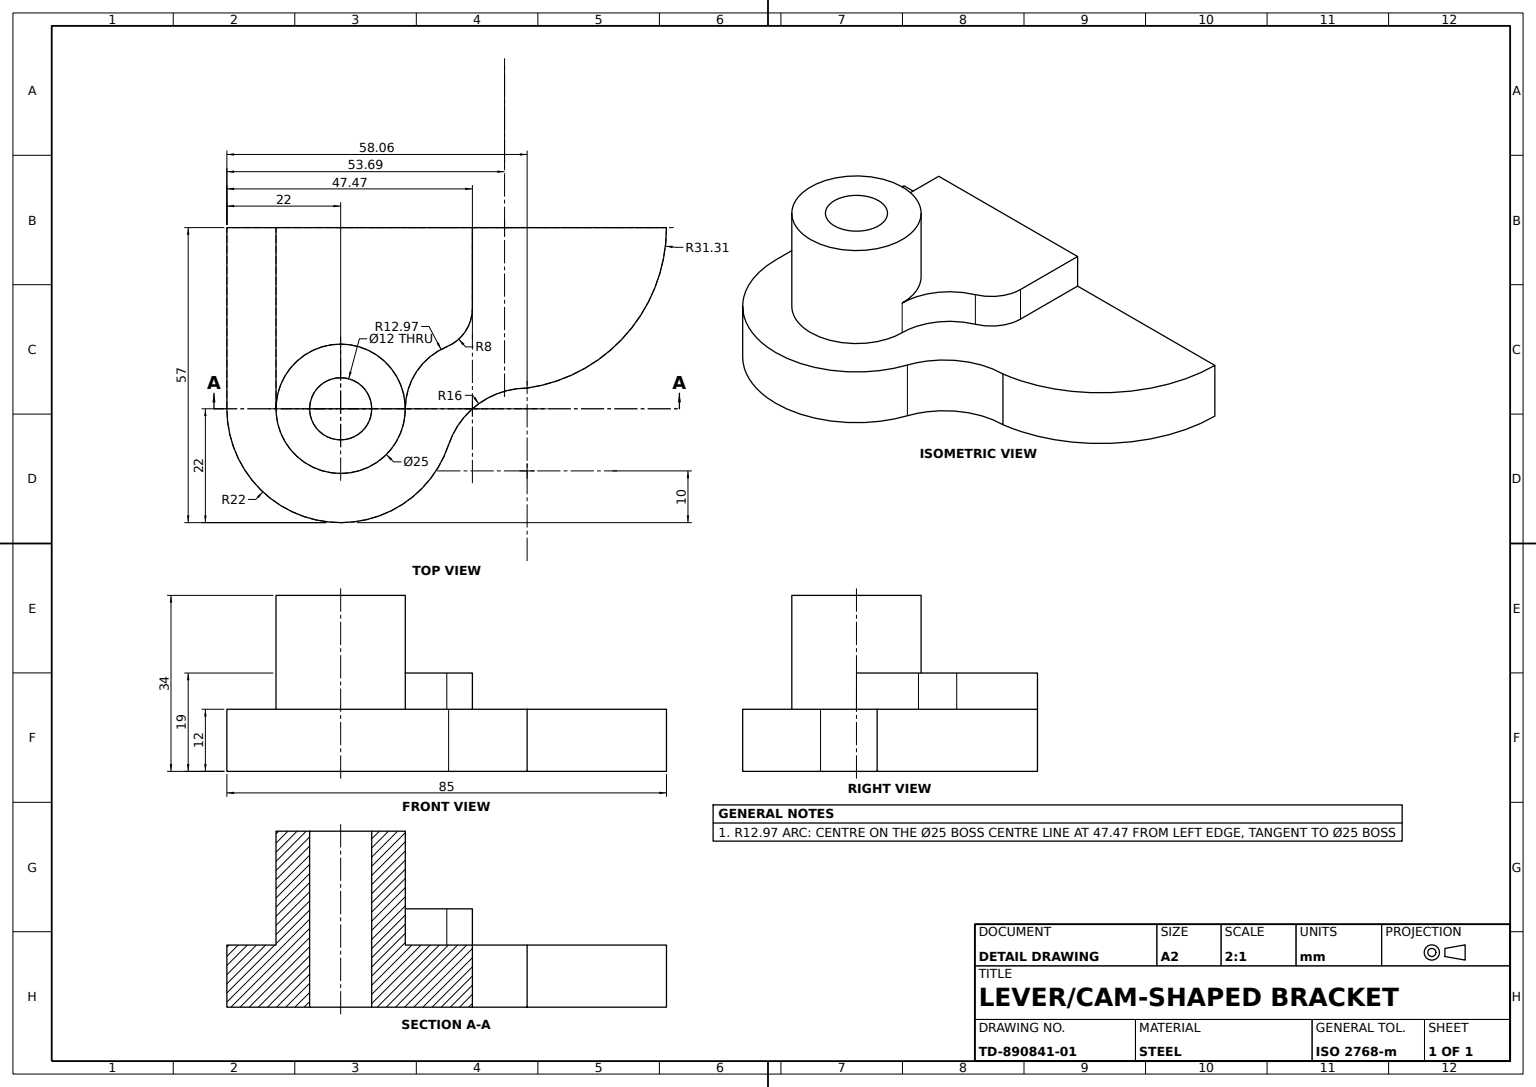
from build123d import *

# Parameters (mm, degrees)
BASE_PLATE_12MM_DEPTH = 12
RAISED_PAD_19MM_DEPTH = 19
HUB_PROFILE_R         = 12.5
HUB_PROFILE_R_2       = 6
HUB_BOSS_34MM_DEPTH   = 34


with BuildPart() as part:
    # Base Plate Profile → Base Plate 12mm (new body)
    with BuildSketch(Plane(origin=(0, 0, 0), x_dir=(1, 0, 0), z_dir=(0, 1, 0))):
        with BuildLine():
            Line((-12.5, 35), (-22, 35))
            Line((-22, 35), (-22, 0))
            ThreePointArc((-22, 0), (-3.518993252, -21.716737473), (20.874244226, -6.947368421))
            ThreePointArc((20.874244226, -6.947368421), (26.697150325, 0.97771369), (36.055512755, 4))
            ThreePointArc((36.055512755, 4), (55.322416794, 14.463414397), (63, 35))
            Line((63, 35), (25.47250751, 35))
            Line((25.47250751, 35), (25.47250751, 19.386749889))
            ThreePointArc((25.47250751, 19.386749889), (24.121301121, 14.937756348), (20.524121628, 11.991639932))
            ThreePointArc((20.524121628, 11.991639932), (14.69106688, 7.214325266), (12.5, 0))
            ThreePointArc((12.5, 0), (0, -12.5), (-12.5, 0))
            Line((-12.5, 0), (-12.5, 35))
        make_face()
    extrude(amount=BASE_PLATE_12MM_DEPTH)

    # Raised Pad Profile → Raised Pad 19mm (add)
    with BuildSketch(Plane(origin=(0, 0, 0), x_dir=(1, 0, 0), z_dir=(0, 1, 0))):
        with BuildLine():
            ThreePointArc((20.524121628, 11.991639932), (24.121301121, 14.937756348), (25.47250751, 19.386749889))
            Line((25.47250751, 19.386749889), (25.47250751, 35))
            Line((25.47250751, 35), (0, 35))
            Line((0, 35), (0, 12.5))
            ThreePointArc((0, 12.5), (8.838834765, 8.838834765), (12.5, 0))
            ThreePointArc((12.5, 0), (14.69106688, 7.214325266), (20.524121628, 11.991639932))
        make_face()
        with BuildLine():
            Line((0, 12.5), (0, 35))
            Line((0, 35), (-12.5, 35))
            Line((-12.5, 35), (-12.5, 0))
            ThreePointArc((-12.5, 0), (-8.838834765, 8.838834765), (0, 12.5))
        make_face()
    extrude(amount=RAISED_PAD_19MM_DEPTH)

    # Hub Profile → Hub Boss 34mm (add)
    with BuildSketch(Plane(origin=(0, 0, 0), x_dir=(1, 0, 0), z_dir=(0, 1, 0))):
        Circle(HUB_PROFILE_R)
        with Locations(Location((0, 0, 0), (0, 0, 270))):
            Circle(HUB_PROFILE_R_2, mode=Mode.SUBTRACT)
    extrude(amount=HUB_BOSS_34MM_DEPTH)


solid = part.part
